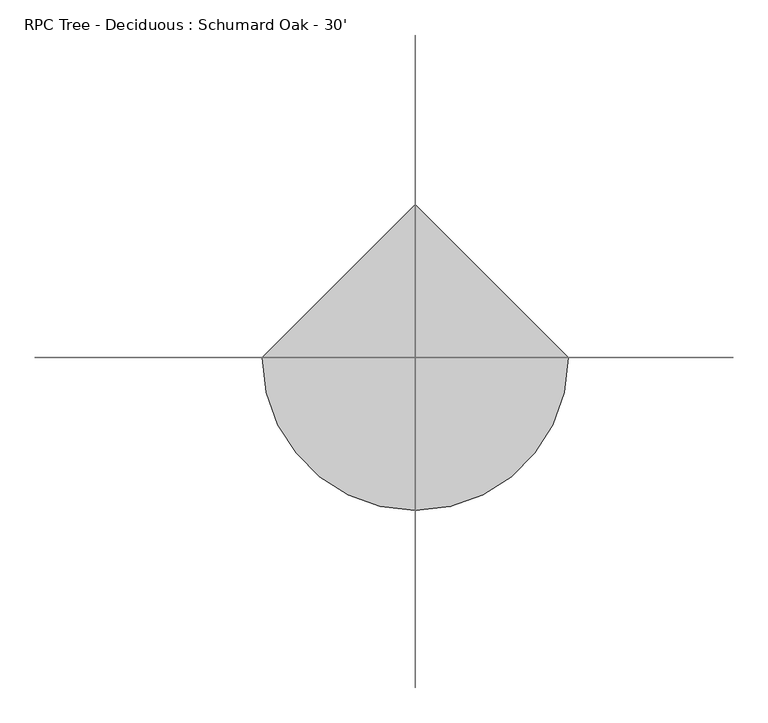
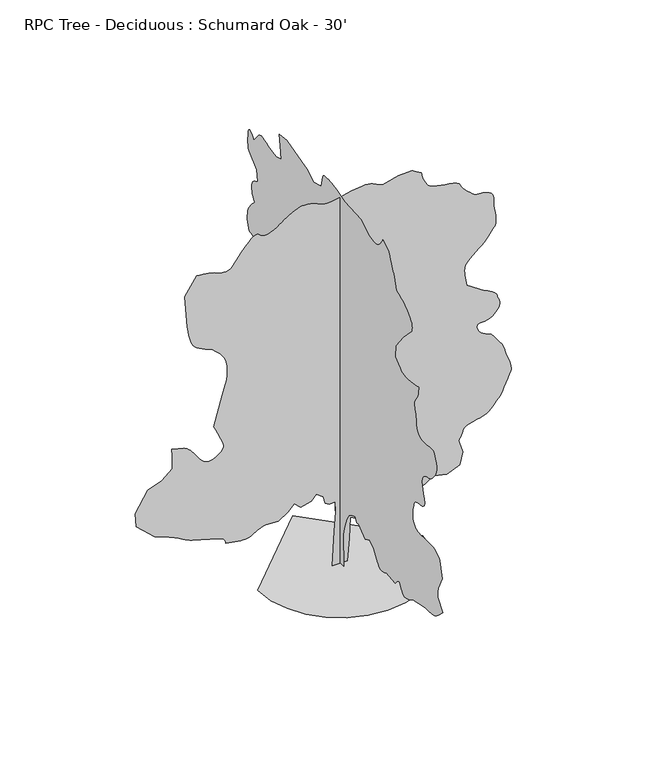
"""IFC4 building model written with IfcOpenShell, lengths in millimetres: geographic element geometry, RPC Tree - Deciduous : Schumard Oak - 30'."""

from ifc_helpers import new_model, si_unit, origin, place, context, project, spatial, triangles, source, transform, mapped, element, save


def rpc_tree_deciduous_schumard_oak_30_cf07c7db(model_context):
    return source(origin(), model_context, "Body", "Tessellation", [
        triangles([(-0.0016958, 164.6246354, 0.0086022), (-0.0016958, -151.6104316, 0.0086022), (-0.0016958, -124.1113561, 783.7227293), (-0.0016958, -179.1089983, 1017.4612965), (-0.0016958, -261.6049622, 1237.4509209), (-0.0016958, -357.8507226, 1388.6927067), (-0.0016958, -467.8454985, 1457.4403999), (-0.0016958, -605.3383779, 1512.436607), (-0.0016958, -660.3370193, 1388.6927067), (-0.0016958, -756.5828161, 1416.1908829), (-0.0016958, -866.5775557, 1306.195998), (-0.0016958, -1017.8194868, 1209.9502739), (-0.0016958, -1196.5619196, 1292.4469826), (-0.0016958, -1361.5527935, 1182.452243), (-0.0016958, -1471.5476784, 989.9607222), (-0.0016958, -1498.1643677, 951.9597713), (-0.0016958, -1525.3829098, 915.7621988), (-0.0016958, -1553.8031227, 883.1739264), (-0.0016958, -1584.0290394, 855.9959341), (-0.0016958, -1616.658007, 836.0340712), (-0.0016958, -1652.2942039, 825.0891724), (-0.0016958, -1691.5371574, 824.9697756), (-0.0016958, -1729.1774471, 831.662681), (-0.0016958, -1760.3255459, 839.8008471), (-0.0016958, -1786.0582775, 849.1404659), (-0.0016958, -1807.4654011, 859.4426714), (-0.0016958, -1825.6238857, 870.4663445), (-0.0016958, -1841.6182583, 881.9725462), (-0.0016958, -1856.5307201, 893.7149254), (-0.0016958, -2214.0131149, 852.4678791), (-0.0016958, -2249.2480282, 893.1561659), (-0.0016958, -2283.7616192, 930.4738735), (-0.0016958, -2316.8324203, 961.0605967), (-0.0016958, -2347.7391094, 981.54314), (-0.0016958, -2375.7578934, 988.5586275), (-0.0016958, -2400.1697754, 978.7389507), (-0.0016958, -2420.2535786, 948.7136032), (-0.0016958, -2440.416156, 905.5412384), (-0.0016958, -2465.389341, 860.9260838), (-0.0016958, -2494.9323051, 818.4750412), (-0.0016958, -2528.8058189, 781.7974108), (-0.0016958, -2566.7735596, 754.4999491), (-0.0016958, -2608.5820541, 740.1896307), (-0.0016958, -2653.9973053, 742.4730669), (-0.0016958, -2699.5395836, 755.8614212), (-0.0016958, -2742.1861084, 772.1352098), (-0.0016958, -2782.4196991, 790.8169184), (-0.0016958, -2820.7484642, 811.421402), (-0.0016958, -2857.6293526, 833.4686754), (-0.0016958, -2893.5448929, 856.475992), (-0.0016958, -2928.9779045, 879.96591), (-0.0016958, -3423.9482735, 976.2117067), (-0.0016958, -3485.6956673, 976.3335743), (-0.0016958, -3546.579451, 977.174366), (-0.0016958, -3605.7868835, 979.4603456), (-0.0016958, -3662.4543549, 983.9078939), (-0.0016958, -3715.7688332, 991.2459635), (-0.0016958, -3764.8925789, 1002.1882462), (-0.0016958, -3808.9361115, 1017.4612965), (-0.0016958, -3851.3797417, 1039.546649), (-0.0016958, -3896.0075409, 1069.5719965), (-0.0016958, -3942.4134293, 1106.2115479), (-0.0016958, -3990.2924835, 1148.1393665), (-0.0016958, -4039.2383331, 1194.0371464), (-0.0016958, -4088.8951859, 1242.5817123), (-0.0016958, -4138.9334106, 1292.4469826), (-0.0016958, -3946.4265564, 1512.436607), (-0.0016958, -3940.7114983, 1553.6455742), (-0.0016958, -3935.9362083, 1594.6132771), (-0.0016958, -3933.0916145, 1635.0983059), (-0.0016958, -3933.1169037, 1674.8646286), (-0.0016958, -3937.0032944, 1713.6657486), (-0.0016958, -3945.7152626, 1751.2679592), (-0.0016958, -3960.1934486, 1787.4247639), (-0.0016958, -4111.425206, 2103.6601124), (-0.0016958, -4015.1842781, 2488.640538), (-0.0016958, -4007.6405525, 2499.2628548), (-0.0016958, -3985.1869812, 2526.4815422), (-0.0016958, -3948.0776184, 2563.3191193), (-0.0016958, -3896.5156494, 2602.8164177), (-0.0016958, -3830.780127, 2637.9697952), (-0.0016958, -3751.1003975, 2661.820665), (-0.0016958, -3657.7046448, 2667.3831161), (-0.0016958, -3553.6406479, 2663.0650658), (-0.0016958, -3446.4524231, 2661.3634254), (-0.0016958, -3343.1000107, 2661.617189), (-0.0016958, -3250.5928665, 2663.0650658), (-0.0016958, -3175.8660324, 2664.970182), (-0.0016958, -3125.9298363, 2666.6718224), (-0.0016958, -3107.7178665, 2667.3831161), (-0.0016958, -3097.049913, 2674.6474983), (-0.0016958, -3069.5669975, 2695.1200859), (-0.0016958, -3031.9495262, 2726.9207611), (-0.0016958, -2990.9793526, 2768.0688309), (-0.0016958, -2953.3874611, 2816.7097572), (-0.0016958, -2925.9045456, 2870.8625565), (-0.0016958, -2915.2365921, 2928.622403), (-0.0016958, -2917.2431557, 2986.3310898), (-0.0016958, -2922.8564758, 3041.9064766), (-0.0016958, -2931.4672874, 3095.6529053), (-0.0016958, -2942.4907425, 3147.977037), (-0.0016958, -2955.3178665, 3199.2087936), (-0.0016958, -2969.3385223, 3249.7039673), (-0.0016958, -2983.9690247, 3299.8436394), (-0.0016958, -2996.0086967, 3314.52472), (-0.0016958, -3009.4706657, 3328.8250099), (-0.0016958, -3025.8280975, 3342.414006), (-0.0016958, -3046.5038704, 3354.9362068), (-0.0016958, -3072.9705688, 3365.9852417), (-0.0016958, -3106.6510712, 3375.2561874), (-0.0016958, -3148.9673836, 3382.3429642), (-0.0016958, -3200.1485619, 3386.6863037), (-0.0016958, -3255.4443146, 3391.740937), (-0.0016958, -3308.7843727, 3403.2725006), (-0.0016958, -3354.1996239, 3427.0722107), (-0.0016958, -3385.6703773, 3468.9315742), (-0.0016958, -3397.1766518, 3534.5906479), (-0.0016958, -3382.6984657, 3629.8406479), (-0.0016958, -3353.0819595, 3737.5114014), (-0.0016958, -3325.8786781, 3836.2667107), (-0.0016958, -3305.152327, 3925.6746254), (-0.0016958, -3294.9921913, 4005.2023293), (-0.0016958, -3299.5387161, 4074.3920013), (-0.0016958, -3322.8306084, 4132.761113), (-0.0016958, -3368.9571533, 4179.8018463), (-0.0016958, -3425.5228867, 4212.7710548), (-0.0016958, -3477.9993347, 4232.964299), (-0.0016958, -3527.3262657, 4246.1975029), (-0.0016958, -3574.5193153, 4258.2118858), (-0.0016958, -3620.493544, 4274.8233719), (-0.0016958, -3666.2390076, 4301.7473099), (-0.0016958, -3712.6954742, 4344.8004959), (-0.0016958, -3760.0411308, 4399.562851), (-0.0016958, -3805.2023277, 4457.9322533), (-0.0016958, -3844.3694138, 4520.1368866), (-0.0016958, -3873.6809967, 4586.4308052), (-0.0016958, -3889.2765564, 4657.068354), (-0.0016958, -3887.295282, 4732.2777168), (-0.0016958, -3863.9272316, 4812.2879494), (-0.0016958, -3835.7077332, 4887.9545517), (-0.0016958, -3816.632444, 4949.7019455), (-0.0016958, -3799.0047409, 4996.9967331), (-0.0016958, -3775.1032928, 5029.3819656), (-0.0016958, -3737.2573471, 5046.3745331), (-0.0016958, -3677.7705711, 5047.4919067), (-0.0016958, -3588.9466324, 5032.2771378), (-0.0016958, -3483.5620766, 5015.437468), (-0.0016958, -3382.266806, 5012.0591858), (-0.0016958, -3289.150106, 5022.1684525), (-0.0016958, -3208.3018433, 5045.7396881), (-0.0016958, -3143.7860138, 5082.7728928), (-0.0016958, -3099.7421906, 5133.2930649), (-0.0016958, -3080.2096619, 5197.2507889), (-0.0016958, -3073.5295464, 5265.5768509), (-0.0016958, -3065.4015541, 5329.5339935), (-0.0016958, -3056.0541595, 5389.9099594), (-0.0016958, -3045.7417076, 5447.3901718), (-0.0016958, -3034.7182526, 5502.7112137), (-0.0016958, -3023.2119781, 5556.5846695), (-0.0016958, -3011.4772293, 5609.7471222), (-0.0016958, -3000.047113, 5648.0755966), (-0.0016958, -2990.8014565, 5686.505809), (-0.0016958, -2985.8485611, 5725.1900757), (-0.0016958, -2987.423465, 5764.2295532), (-0.0016958, -2997.6341789, 5803.7521408), (-0.0016958, -3018.6907425, 5843.8839935), (-0.0016958, -3052.7267464, 5884.7274307), (-0.0016958, -3089.125106, 5934.8418137), (-0.0016958, -3116.6080215, 5997.6815826), (-0.0016958, -3136.4198936, 6065.8297485), (-0.0016958, -3149.7295464, 6131.8187439), (-0.0016958, -3157.7558006, 6188.1815826), (-0.0016958, -3161.6674805, 6227.450116), (-0.0016958, -3162.7089867, 6242.2073547), (-0.0016958, -3142.4395844, 6237.6861191), (-0.0016958, -3088.0074417, 6226.1798447), (-0.0016958, -3009.0387154, 6210.8383392), (-0.0016958, -2915.160434, 6194.7602509), (-0.0016958, -2815.9731743, 6181.0948059), (-0.0016958, -2721.1295448, 6172.9418152), (-0.0016958, -2640.2304131, 6173.4749222), (-0.0016958, -2571.9299309, 6185.3619873), (-0.0016958, -2507.9599983, 6208.094902), (-0.0016958, -2447.5915901, 6239.8452896), (-0.0016958, -2390.1089069, 6278.808609), (-0.0016958, -2334.7901905, 6323.1826447), (-0.0016958, -2280.9167347, 6371.1634369), (-0.0016958, -2227.7621304, 6420.9476074), (-0.0016958, -2241.5111458, 6709.6945175), (-0.0016958, -2543.9897758, 7094.6826462), (-0.0016958, -2887.7283875, 7452.1625702), (-0.0016958, -2893.1132332, 7496.4860275), (-0.0016958, -2895.3482712, 7541.6722229), (-0.0016958, -2891.335144, 7588.5356415), (-0.0016958, -2877.9493332, 7637.9128601), (-0.0016958, -2852.0666107, 7690.6689423), (-0.0016958, -2810.5377502, 7747.6160477), (-0.0016958, -2750.2379425, 7809.6424942), (-0.0016958, -2679.5242355, 7869.2562973), (-0.0016958, -2608.8108192, 7919.4724182), (-0.0016958, -2538.10467, 7961.8901779), (-0.0016958, -2467.3935791, 7998.0344833), (-0.0016958, -2396.6824883, 8029.5052368), (-0.0016958, -2325.9712521, 8057.8517624), (-0.0016958, -2255.2601612, 8084.6233841), (-0.0016958, -2234.6175259, 8155.1336151), (-0.0016958, -2213.8530956, 8224.4503143), (-0.0016958, -2192.8472557, 8291.3537888), (-0.0016958, -2171.4808273, 8354.651088), (-0.0016958, -2149.6341957, 8413.1219376), (-0.0016958, -2127.1881821, 8465.5983856), (-0.0016958, -2104.0183754, 8510.8607391), (-0.0016958, -2078.3235775, 8560.2129593), (-0.0016958, -2049.9822842, 8621.0970337), (-0.0016958, -2021.4021973, 8686.5529221), (-0.0016958, -1994.9862225, 8749.5955856), (-0.0016958, -1973.1395908, 8803.2917267), (-0.0016958, -1958.2679695, 8840.6039841), (-0.0016958, -1952.7738281, 8854.5996414), (-0.0016958, -1719.0353336, 8992.089505), (-0.0016958, -1707.0516174, 8968.3915329), (-0.0016958, -1693.863905, 8943.9819763), (-0.0016958, -1678.2681999, 8918.1248337), (-0.0016958, -1659.0683544, 8890.1085205), (-0.0016958, -1635.057756, 8859.1970352), (-0.0016958, -1605.0324085, 8824.678212), (-0.0016958, -1567.7934025, 8785.841629), (-0.0016958, -1522.9369835, 8752.2122864), (-0.0016958, -1471.5882282, 8732.2983856), (-0.0016958, -1414.8268673, 8723.7896027), (-0.0016958, -1353.7372822, 8724.4244476), (-0.0016958, -1289.3990582, 8731.9175949), (-0.0016958, -1222.896722, 8743.9825562), (-0.0016958, -1155.3123299, 8758.3334244), (-0.0016958, -852.8259968, 8964.5813004), (-0.0016958, -192.8582863, 9005.8311081), (-0.0016958, -107.5965211, 9029.2756073), (-0.0016958, -23.416737, 9052.008522), (-0.0016958, 58.5983536, 9073.2938507), (-0.0016958, 137.366361, 9092.4200089), (-0.0016958, 211.8051857, 9108.6504135), (-0.0016958, 280.8327856, 9121.2740616), (-0.0016958, 343.3650879, 9129.57995), (-0.0016958, 405.0185557, 9135.9045639), (-0.0016958, 469.5549508, 9141.5181747), (-0.0016958, 533.1311937, 9144.0075577), (-0.0016958, 591.8966838, 9140.9594879), (-0.0016958, 642.0033274, 9129.9863205), (-0.0016958, 679.6029219, 9108.6504135), (-0.0016958, 700.8500261, 9074.5891205), (-0.0016958, 769.5952486, 8799.5832321), (-0.0016958, 1072.081509, 8717.1091965), (-0.0016958, 1347.0698112, 8882.0822662), (-0.0016958, 1690.8031906, 8964.5813004), (-0.0016958, 2144.5313095, 9102.0717453), (-0.0016958, 2447.0174973, 9060.8225189), (-0.0016958, 2419.5169956, 8799.5832321), (-0.0016958, 2364.5209339, 8497.1197174), (-0.0016958, 2584.5030006, 8428.361705), (-0.0016958, 2804.4924797, 8469.6115128), (-0.0016958, 2889.5570549, 8501.5647949), (-0.0016958, 2972.3357231, 8530.7490601), (-0.0016958, 3050.5425774, 8554.3964539), (-0.0016958, 3121.8911293, 8569.7385406), (-0.0016958, 3184.1210518, 8574.0307205), (-0.0016958, 3234.8958595, 8564.480722), (-0.0016958, 3271.9799332, 8538.3439453), (-0.0016958, 3478.2280998, 8290.8712601), (-0.0016958, 3525.090937, 8345.6591949), (-0.0016958, 3570.2521339, 8393.3603531), (-0.0016958, 3612.0606285, 8426.8885391), (-0.0016958, 3648.8144897, 8439.1058167), (-0.0016958, 3678.8373665, 8422.9515701), (-0.0016958, 3700.4526169, 8371.313443), (-0.0016958, 3711.9588913, 8277.1046585), (-0.0016958, 3715.4389114, 8172.4819748), (-0.0016958, 3714.6005905, 8091.684581), (-0.0016958, 3710.155513, 8030.6987686), (-0.0016958, 3702.8149727, 7985.6137299), (-0.0016958, 3693.3152618, 7952.4163376), (-0.0016958, 3682.3679649, 7927.1684601), (-0.0016958, 3670.7093742, 7905.8831314), (-0.0016958, 3354.4789673, 7644.6438446), (-0.0016958, 3326.9707626, 7355.921933), (-0.0016958, 3370.9384277, 7337.989888), (-0.0016958, 3413.6102417, 7318.6346741), (-0.0016958, 3453.615358, 7296.384288), (-0.0016958, 3489.6326363, 7269.8161423), (-0.0016958, 3520.3920959, 7237.4564896), (-0.0016958, 3544.5220184, 7197.8833237), (-0.0016958, 3560.7018448, 7149.674057), (-0.0016958, 3566.8994316, 7096.6389221), (-0.0016958, 3562.9624626, 7043.6032059), (-0.0016958, 3550.618158, 6990.568071), (-0.0016958, 3531.5425781, 6937.5329361), (-0.0016958, 3507.4126556, 6884.4978012), (-0.0016958, 3479.904451, 6831.4626663), (-0.0016958, 3450.7198952, 6778.4269501), (-0.0016958, 3494.7381386, 6734.2313919), (-0.0016958, 3537.6640068, 6689.8829361), (-0.0016958, 3578.4309952, 6645.3060059), (-0.0016958, 3615.9470192, 6600.3732834), (-0.0016958, 3649.1447021, 6554.9580322), (-0.0016958, 3676.9322502, 6508.9329346), (-0.0016958, 3698.2175789, 6462.1968338), (-0.0016958, 3713.4829262, 6416.6548462), (-0.0016958, 3724.4305138, 6374.0080307), (-0.0016958, 3731.7710541, 6333.77444), (-0.0016958, 3736.2161316, 6295.4459656), (-0.0016958, 3738.5020386, 6258.5650772), (-0.0016958, 3739.3400688, 6222.6492462), (-0.0016958, 3739.4670959, 6187.2165253), (-0.0016958, 3656.9680618, 5953.4854431), (-0.0016958, 3618.6901657, 5947.3387253), (-0.0016958, 3580.5140076, 5939.7694199), (-0.0016958, 3542.591613, 5929.304361), (-0.0016958, 3505.0250107, 5914.5215424), (-0.0016958, 3467.9665169, 5893.9477982), (-0.0016958, 3431.4664192, 5866.1599594), (-0.0016958, 3395.728775, 5829.7366013), (-0.0016958, 3363.165937, 5786.4799393), (-0.0016958, 3335.6830215, 5739.6171021), (-0.0016958, 3312.3911293, 5689.7567734), (-0.0016958, 3292.4522301, 5637.4838013), (-0.0016958, 3275.0532921, 5583.4068695), (-0.0016958, 3259.3559944, 5528.1364059), (-0.0016958, 3244.4717285, 5472.2566772), (-0.0016958, 3212.2896812, 5428.0349579), (-0.0016958, 3181.4287743, 5383.7120819), (-0.0016958, 3153.2092758, 5339.1351517), (-0.0016958, 3128.9523262, 5294.1768494), (-0.0016958, 3110.0037735, 5248.7615982), (-0.0016958, 3097.6341797, 5202.7620804), (-0.0016958, 3093.2399712, 5156.026561), (-0.0016958, 3106.9812836, 4784.7797447), (-0.0016958, 3139.1630402, 4781.5284897), (-0.0016958, 3170.049527, 4776.4738564), (-0.0016958, 3198.2690254, 4767.8377556), (-0.0016958, 3222.5006859, 4753.7662308), (-0.0016958, 3241.4745277, 4732.4809021), (-0.0016958, 3253.8188324, 4702.1533928), (-0.0016958, 3258.2383301, 4661.0306122), (-0.0016958, 3257.0192184, 4613.5073502), (-0.0016958, 3253.6665161, 4565.2219254), (-0.0016958, 3248.4848557, 4516.377523), (-0.0016958, 3241.8808983, 4467.0253029), (-0.0016958, 3234.1845657, 4417.3175812), (-0.0016958, 3225.7516502, 4367.3810944), (-0.0016958, 3216.988813, 4317.2922913), (-0.0016958, 3203.2219208, 4042.311692), (-0.0016958, 3464.4612076, 4056.0785843), (-0.0016958, 3753.208699, 4111.0694138), (-0.0016958, 3814.6511696, 4090.2669044), (-0.0016958, 3873.5792587, 4068.37202), (-0.0016958, 3927.4527145, 4044.3182556), (-0.0016958, 3973.7568649, 4017.0132362), (-0.0016958, 4009.9520393, 3985.3901665), (-0.0016958, 4033.523275, 3948.3569618), (-0.0016958, 4041.9306107, 3904.8212471), (-0.0016958, 4039.5429657, 3849.6778107), (-0.0016958, 4032.8119812, 3780.081768), (-0.0016958, 4022.448951, 3698.4716331), (-0.0016958, 4009.2407455, 3607.2347603), (-0.0016958, 3993.8483711, 3508.7840836), (-0.0016958, 3977.00812, 3405.5078293), (-0.0016958, 3959.4568657, 3299.8436394), (-0.0016958, 3835.7077332, 2969.87192), (-0.0016958, 3768.1185448, 2931.9498161), (-0.0016958, 3701.6211502, 2896.3136192), (-0.0016958, 3637.2829262, 2865.2492363), (-0.0016958, 3576.1959572, 2841.0431557), (-0.0016958, 3519.4267479, 2825.9554138), (-0.0016958, 3468.0679642, 2822.3233681), (-0.0016958, 3423.2113998, 2832.3817657), (-0.0016958, 3038.248851, 2997.3548355), (-0.0016958, 2653.2607224, 2873.6312828), (-0.0016958, 2378.2699493, 2681.1244286), (-0.0016958, 2103.2842632, 2268.651059), (-0.0016958, 2076.6675739, 2227.6428062), (-0.0016958, 2049.4488865, 2188.0796688), (-0.0016958, 2021.0263481, 2151.4021111), (-0.0016958, 1990.8027569, 2119.0526321), (-0.0016958, 1958.1739346, 2092.4764927), (-0.0016958, 1922.5377377, 2073.1141571), (-0.0016958, 1883.2946388, 2062.4105953), (-0.0016958, 1844.1303143, 2058.8443886), (-0.0016958, 1807.3715115, 2059.123732), (-0.0016958, 1770.371299, 2062.0498615), (-0.0016958, 1730.4881229, 2066.4186356), (-0.0016958, 1685.070401, 2071.0288193), (-0.0016958, 1631.4762886, 2074.6762711), (-0.0016958, 1567.0592903, 2076.1596107), (-0.0016958, 1497.9510086, 2070.950045), (-0.0016958, 1431.730632, 2056.3577671), (-0.0016958, 1367.9130157, 2033.9498325), (-0.0016958, 1306.020718, 2005.2883553), (-0.0016958, 1245.5712101, 1971.9382107), (-0.0016958, 1186.0844341, 1935.4612221), (-0.0016958, 1127.0801868, 1897.4196487), (-0.0016958, 1044.5834782, 1663.6810089), (-0.0016958, 810.8448383, 1402.4418674), (-0.0016958, 778.5741337, 1367.4862976), (-0.0016958, 741.256426, 1333.2546661), (-0.0016958, 699.7273476, 1299.622562), (-0.0016958, 654.8303061, 1266.4729866), (-0.0016958, 607.408455, 1233.6815289), (-0.0016958, 558.3051295, 1201.1339516), (-0.0016958, 508.3585416, 1168.7032276), (-0.0016958, 425.8618329, 1457.4403999), (-0.0016958, 288.3689717, 1649.9293774), (-0.0016958, 233.3715837, 1526.1856224), (-0.0016958, 192.1232112, 1333.696645), (-0.0016958, 178.3741776, 989.9607222), (-0.0016958, 150.8753565, 508.7344634), (170.3625119, 0.000436, 0.0217742), (-187.1199193, 0.000436, 0.0217742), (-132.1230309, 0.000387, 824.9824928), (-104.6242098, 0.0003581, 1306.2087879), (-118.3734886, 0.0003434, 1553.698914), (-255.8671038, 0.0003442, 1539.9498985), (-352.1128461, 0.000341, 1594.9459602), (-393.359965, 0.0003302, 1773.6885384), (-558.3534187, 0.0003237, 1883.6832779), (-668.3482309, 0.000331, 1759.9395229), (-915.8358135, 0.0003352, 1691.1918297), (-1067.0802881, 0.0003271, 1828.6846001), (-1218.3221466, 0.000336, 1677.4428143), (-1438.311771, 0.0003442, 1539.9498985), (-1768.2961349, 0.0003434, 1553.698914), (-1933.2869362, 0.0003476, 1484.9512207), (-1968.7250347, 0.0003491, 1458.6138748), (-2004.6407204, 0.0003507, 1433.3612011), (-2041.5189926, 0.000352, 1410.2726395), (-2079.8425255, 0.0003531, 1390.4301006), (-2120.0889061, 0.0003541, 1374.915786), (-2162.738047, 0.0003547, 1364.8142223), (-2208.2752384, 0.0003549, 1361.2074657), (-2259.0244663, 0.0003549, 1362.8101295), (-2316.2658852, 0.0003547, 1367.3008438), (-2378.9175842, 0.0003541, 1374.1944637), (-2445.902449, 0.0003536, 1383.0132568), (-2516.1310112, 0.0003531, 1393.2749851), (-2588.5161278, 0.0003523, 1404.4991547), (-2661.9982704, 0.0003518, 1416.2061436), (-2665.4018417, 0.0003499, 1445.5887978), (-2671.5741394, 0.0003481, 1474.4889233), (-2683.2835991, 0.0003465, 1502.428933), (-2703.2986565, 0.0003449, 1528.9262981), (-2734.3630394, 0.0003434, 1553.4981995), (-2779.2448929, 0.0003421, 1575.6648697), (-2840.7382324, 0.000341, 1594.9459602), (-3445.7158401, 0.0003302, 1773.6885384), (-3495.0936401, 0.0003295, 1789.3602562), (-3547.8494316, 0.0003281, 1811.5293972), (-3602.2815742, 0.0003266, 1838.265556), (-3656.7140076, 0.0003247, 1867.6482101), (-3709.469799, 0.0003229, 1897.7523319), (-3758.8728882, 0.0003213, 1926.6550735), (-3803.1957642, 0.0003197, 1952.4285004), (-3850.8716331, 0.0003182, 1977.2011162), (-3910.0790657, 0.0003166, 2004.1403149), (-3978.8876564, 0.0003148, 2032.8804211), (-4055.4181595, 0.0003132, 2063.0657879), (-4137.7140083, 0.0003113, 2094.3332108), (-4223.8456696, 0.0003092, 2126.3194851), (-4311.9327347, 0.0003074, 2158.668964), (-4738.1450912, 0.0002835, 2557.4011665), (-4765.6532959, 0.0002638, 2887.3725952), (-4476.9060951, 0.000236, 3354.8600487), (-4146.9343758, 0.0002287, 3478.6088905), (-3899.4364014, 0.0002163, 3684.8570572), (-3899.4364014, 0.0001977, 4001.0874641), (-3913.2032936, 0.0001877, 4166.0858231), (-3624.4558022, 0.0001919, 4097.3281013), (-3591.9438332, 0.0001932, 4076.3729851), (-3558.8475975, 0.0001945, 4053.3607269), (-3524.5322502, 0.0001961, 4026.2588928), (-3488.4135246, 0.0001979, 3993.03563), (-3449.8815742, 0.0002006, 3951.6082169), (-3408.3524231, 0.0002037, 3899.9953789), (-3363.216806, 0.0002074, 3836.0888145), (-3317.4713425, 0.0002113, 3768.956575), (-3273.4275192, 0.000215, 3709.7491425), (-3229.3839867, 0.0002179, 3659.6856285), (-3183.6385231, 0.0002203, 3619.9601463), (-3134.5403572, 0.0002221, 3591.765937), (-3080.387558, 0.0002229, 3576.3482735), (-3019.4781944, 0.0002229, 3574.8495277), (-2952.9046417, 0.0002221, 3590.0895859), (-2885.848851, 0.0002203, 3620.9507835), (-2822.8567657, 0.0002176, 3662.8860146), (-2768.5513596, 0.0002147, 3711.2984665), (-2727.4541588, 0.0002119, 3761.6413239), (-2704.1622665, 0.000209, 3809.3427727), (-2703.2480782, 0.0002066, 3849.8304176), (-2719.4531937, 0.000204, 3893.6198959), (-2743.5831161, 0.0002006, 3952.5479851), (-2774.3172867, 0.0001961, 4024.0997223), (-2810.3598541, 0.0001914, 4105.735437), (-2850.3649704, 0.0001861, 4194.9657463), (-2893.0114952, 0.0001803, 4289.2506889), (-2936.9788696, 0.0001746, 4386.0755928), (-2744.4975952, 0.0001328, 5087.2685486), (-2718.1576332, 0.0001281, 5166.6433548), (-2692.9100464, 0.0001234, 5244.9263672), (-2669.8216301, 0.0001189, 5321.050209), (-2649.9841782, 0.0001145, 5393.948085), (-2634.4647766, 0.0001105, 5462.477623), (-2624.3555099, 0.0001066, 5525.6220245), (-2620.7487534, 0.0001034, 5582.263916), (-2621.6885216, 0.0001, 5637.5343796), (-2624.7618805, 9.66e-05, 5696.1831253), (-2630.5022278, 9.29e-05, 5756.5079315), (-2639.366803, 8.93e-05, 5816.8333191), (-2651.8128456, 8.58e-05, 5875.4820648), (-2668.3737534, 8.24e-05, 5930.7525284), (-2689.5064751, 7.95e-05, 5980.9936478), (-2716.6844673, 7.67e-05, 6027.7297485), (-2750.3649696, 7.4e-05, 6073.7542648), (-2789.4303177, 7.14e-05, 6119.169516), (-2832.8390053, 6.85e-05, 6164.1022385), (-2879.4986572, 6.59e-05, 6208.6791687), (-2928.3430595, 6.33e-05, 6253.002626), (-2978.2286774, 6.06e-05, 6297.223764), (-3057.4511673, 5.88e-05, 6329.6851547), (-3134.6165154, 5.67e-05, 6362.5273361), (-3207.6922874, 5.49e-05, 6396.0805206), (-3274.6213417, 5.28e-05, 6430.7010818), (-3333.3971146, 5.07e-05, 6466.7942276), (-3381.9365936, 4.83e-05, 6504.6657532), (-3418.2076355, 4.59e-05, 6544.7214478), (-3446.7573463, 4.28e-05, 6598.1123749), (-3473.1478867, 3.86e-05, 6670.5027237), (-3496.8717293, 3.36e-05, 6753.9668152), (-3517.4710533, 2.84e-05, 6840.5557159), (-3534.4636208, 2.34e-05, 6922.3181671), (-3547.3669029, 1.94e-05, 6991.3558136), (-3555.7233696, 1.65e-05, 7039.6918167), (-3610.7144897, -2.94e-05, 7809.6424942), (-3335.7086014, -5.49e-05, 8235.8804306), (-3262.2517479, -5.43e-05, 8226.9396973), (-3189.8616898, -5.38e-05, 8217.4146973), (-3119.6305115, -5.3e-05, 8206.6705856), (-3052.6252991, -5.22e-05, 8194.1225143), (-2989.9887154, -5.15e-05, 8179.162381), (-2932.7372681, -5.04e-05, 8161.2041748), (-2881.9880402, -4.91e-05, 8139.6397934), (-2830.4004913, -4.78e-05, 8118.7864151), (-2772.3107231, -4.7e-05, 8104.2064911), (-2711.3504906, -4.65e-05, 8097.069136), (-2651.1018425, -4.67e-05, 8098.5934616), (-2595.1709541, -4.73e-05, 8109.9724182), (-2547.1901619, -4.86e-05, 8132.4262802), (-2510.7589554, -5.07e-05, 8167.1224182), (-2290.7694763, -6.8e-05, 8455.8699097), (-2232.0038773, -7.19e-05, 8523.1291763), (-2174.2011555, -7.59e-05, 8587.3915329), (-2118.3236069, -7.93e-05, 8645.6333267), (-2065.3290218, -8.22e-05, 8694.8588104), (-2016.1850739, -8.45e-05, 8732.0699112), (-1971.8492626, -8.58e-05, 8754.2185593), (-1933.2869362, -8.61e-05, 8758.3590042), (-1902.260923, -8.53e-05, 8748.0212631), (-1877.0081039, -8.43e-05, 8731.181012), (-1853.1982201, -8.32e-05, 8711.4450073), (-1826.5002857, -8.22e-05, 8692.4455856), (-1792.5886929, -8.11e-05, 8677.7900848), (-1747.1302757, -8.09e-05, 8671.0591003), (-1685.7992809, -8.11e-05, 8675.8593887), (-1612.5227943, -8.24e-05, 8696.712767), (-1537.32346, -8.43e-05, 8731.5112244), (-1465.0070892, -8.69e-05, 8773.9795624), (-1400.3895218, -8.95e-05, 8817.9216476), (-1348.2787491, -9.19e-05, 8857.0378647), (-1313.4833439, -9.35e-05, 8885.1047562), (-1300.8163845, -9.42e-05, 8895.8488678), (-1285.3045406, -9.48e-05, 8905.7802383), (-1244.0574944, -9.63e-05, 8931.6123825), (-1185.0100084, -9.84e-05, 8967.2741592), (-1116.1022959, -0.0001008, 9006.7961655), (-1045.2718082, -0.0001029, 9044.1595825), (-980.4534536, -0.0001047, 9073.344429), (-929.5848289, -0.0001055, 9088.3307236), (-881.3222952, -0.0001058, 9091.6578461), (-821.2740709, -0.0001058, 9089.7021515), (-752.8083372, -0.0001053, 9082.2090042), (-679.2905136, -0.0001045, 9068.9505112), (-604.0912156, -0.0001034, 9049.6714554), (-530.573392, -0.0001019, 9024.1189453), (-462.1076583, -0.0001, 8992.089505), (-389.2730779, -9.84e-05, 8965.9533096), (-302.0062388, -9.79e-05, 8956.4283096), (-202.713753, -9.79e-05, 8960.7204895), (-93.8012603, -9.9e-05, 8976.0625763), (22.3266441, -0.0001003, 8999.7099701), (143.2647473, -0.0001021, 9028.8942352), (266.608781, -0.000104, 9060.8475174), (351.7496415, -0.0001047, 9072.3793716), (435.0871056, -0.0001053, 9082.4886383), (514.8177767, -0.0001058, 9089.7021515), (589.1356968, -0.0001058, 9092.597905), (656.2400311, -0.0001058, 9089.7021515), (714.324785, -0.000105, 9079.5928848), (761.584037, -0.000104, 9060.8475174), (801.2284195, -0.0001026, 9038.8767654), (837.987295, -0.0001016, 9019.8011856), (872.3408667, -0.0001005, 9003.1132507), (904.7690472, -9.98e-05, 8988.356012), (935.7570539, -9.9e-05, 8975.0719391), (965.779858, -9.82e-05, 8962.7017639), (995.3226768, -9.74e-05, 8950.8402786), (1352.8050716, -0.0001032, 9047.0809158), (1669.0404202, -0.000104, 9060.8475174), (1889.0325153, -9.66e-05, 8937.0986755), (1892.1974384, -9.48e-05, 8904.5611267), (1896.6881527, -9.27e-05, 8871.1602585), (1903.8228916, -9.06e-05, 8836.0827484), (1914.9278824, -8.85e-05, 8798.4908569), (1931.3210678, -8.58e-05, 8757.5206833), (1954.3308552, -8.32e-05, 8712.3339066), (1985.2757687, -8.03e-05, 8662.118367), (2016.3831722, -7.74e-05, 8616.1438477), (2042.1971489, -7.56e-05, 8582.1842926), (2067.531213, -7.4e-05, 8557.1398911), (2097.1958267, -7.27e-05, 8537.8358368), (2135.9969467, -7.19e-05, 8521.1990616), (2188.7502674, -7.09e-05, 8504.1047562), (2260.2639256, -6.96e-05, 8483.3781143), (2348.4121788, -6.85e-05, 8463.4136353), (2443.5351517, -6.75e-05, 8448.2500259), (2539.1383278, -6.67e-05, 8434.3055283), (2628.7244293, -6.56e-05, 8417.9478058), (2705.8133286, -6.43e-05, 8395.5701019), (2763.9030968, -6.25e-05, 8363.5918213), (2796.4915146, -5.99e-05, 8318.3794647), (2820.5705681, -5.67e-05, 8265.7507004), (2856.206765, -5.36e-05, 8213.8329391), (2901.4696999, -5.04e-05, 8162.5250244), (2954.4286766, -4.75e-05, 8111.6996384), (3013.1535805, -4.44e-05, 8061.2300446), (3075.7137154, -4.15e-05, 8011.0139236), (3140.2298355, -3.83e-05, 7960.8995407), (3230.9333107, -3.78e-05, 7951.6035965), (3317.928582, -3.73e-05, 7939.5386353), (3397.4559952, -3.62e-05, 7921.9362213), (3465.8073463, -3.47e-05, 7896.027919), (3519.2235626, -3.23e-05, 7859.0708725), (3554.0217293, -2.94e-05, 7808.2966461), (3566.4421921, -2.55e-05, 7740.9100616), (3567.2549332, -2.13e-05, 7670.7044632), (3569.4902618, -1.76e-05, 7612.0812973), (3572.9447021, -1.47e-05, 7563.0337097), (3577.3641998, -1.23e-05, 7521.7077438), (3582.4949913, -1.02e-05, 7486.1732849), (3588.1086021, -8.1e-06, 7454.4484772), (3593.9503967, -6.6e-06, 7424.6799454), (3605.4566711, -2.4e-06, 7354.1947128), (3615.2865944, 1.8e-06, 7285.1832275), (3621.7382355, 5.8e-06, 7219.0413345), (3623.1352432, 9.5e-06, 7157.2177826), (3617.8009758, 1.29e-05, 7101.1851563), (3604.0596634, 1.58e-05, 7052.3666245), (3580.2090843, 1.81e-05, 7012.1836121), (3549.779837, 2.05e-05, 6973.6772415), (3516.9376556, 2.31e-05, 6929.6084198), (3480.9965355, 2.6e-05, 6881.221257), (3441.1948952, 2.89e-05, 6829.7098663), (3396.8208595, 3.2e-05, 6776.2933594), (3347.138427, 3.54e-05, 6722.1408508), (3291.4615929, 3.86e-05, 6668.4452911), (3226.8184456, 4.2e-05, 6613.0986694), (3154.6824417, 4.54e-05, 6553.8912369), (3081.1241409, 4.91e-05, 6492.0421051), (3012.1376541, 5.28e-05, 6428.7453873), (2953.7429626, 5.67e-05, 6365.2196136), (2911.9344681, 6.04e-05, 6302.6338989), (2892.7321518, 6.41e-05, 6242.2329346), (2889.6587929, 6.75e-05, 6182.4918137), (2891.6144875, 7.11e-05, 6121.3286865), (2897.7867851, 7.48e-05, 6058.9464478), (2907.3370743, 7.88e-05, 5995.6241501), (2919.4020355, 8.24e-05, 5931.5652695), (2933.1436386, 8.64e-05, 5867.0238602), (2947.7232719, 9.03e-05, 5802.2533951), (3360.2196053, 0.0001066, 5527.2475067), (3376.1959557, 0.0001071, 5520.1357315), (3417.4457634, 0.0001082, 5500.475885), (3473.8591805, 0.00011, 5470.9864059), (3535.3019417, 0.0001121, 5434.2584152), (3591.7153587, 0.0001147, 5392.9830276), (3632.9648758, 0.0001171, 5349.7525269), (3648.9415169, 0.0001197, 5307.2580276), (3657.5267487, 0.0001221, 5267.1511734), (3677.1610153, 0.0001244, 5227.0193207), (3698.7256874, 0.0001271, 5183.5347656), (3713.0765556, 0.0001302, 5133.2930649), (3711.0699921, 0.0001336, 5072.9682587), (3683.5870766, 0.0001381, 4999.1814835), (3621.4586014, 0.0001436, 4908.5282959), (3535.7588905, 0.0001481, 4831.4141075), (3447.6462456, 0.0001504, 4791.5613075), (3363.1403572, 0.0001515, 4775.7881424), (3288.2612068, 0.0001517, 4770.8096672), (3229.0029053, 0.0001523, 4763.4182579), (3191.4110138, 0.0001536, 4740.4312889), (3181.4796432, 0.0001567, 4688.5388168), (3195.7796425, 0.0001604, 4623.8450912), (3225.2438324, 0.0001635, 4569.9716354), (3267.3316704, 0.0001664, 4525.1153618), (3319.528775, 0.0001685, 4487.4723106), (3379.2948944, 0.0001704, 4455.2396851), (3444.1156471, 0.0001722, 4426.6393959), (3511.4510719, 0.0001738, 4399.8169052), (3578.7612076, 0.0001788, 4314.6761719), (3643.3026169, 0.0001838, 4231.3385262), (3702.3068642, 0.0001885, 4151.6079277), (3753.0055138, 0.000193, 4077.2874641), (3792.6548378, 0.0001972, 4010.1805138), (3818.4611115, 0.0002006, 3952.0907455), (3827.6814789, 0.0002032, 3904.8468269), (3838.9084099, 0.0002066, 3848.3063828), (3866.9753014, 0.0002116, 3767.5086983), (3903.4498192, 0.0002171, 3671.7761696), (3939.9240463, 0.0002231, 3570.531768), (3967.9912285, 0.0002289, 3473.1225975), (3979.2178688, 0.0002342, 3388.9469215), (3965.1716331, 0.0002378, 3327.351844), (3932.583506, 0.0002413, 3266.5442184), (3894.7119804, 0.0002462, 3184.3498169), (3852.9799347, 0.000252, 3089.6076347), (3808.8599533, 0.0002578, 2991.2842758), (3763.7496254, 0.0002633, 2898.2440247), (3719.1471153, 0.000268, 2819.4023254), (3676.4497215, 0.0002714, 2763.6493332), (3635.0475975, 0.0002741, 2719.4784828), (3592.6804161, 0.000277, 2671.193058), (3548.3828293, 0.0002798, 2621.4853363), (3501.189489, 0.0002827, 2572.9967262), (3450.1609177, 0.0002854, 2528.3384056), (3394.3317673, 0.0002877, 2490.1773628), (3332.7114006, 0.0002893, 2461.1552971), (3259.8893921, 0.0002906, 2439.6287041), (3175.9677704, 0.0002919, 2420.2688393), (3088.4646812, 0.000293, 2400.1850361), (3004.822403, 0.0002943, 2376.4944763), (2932.457634, 0.0002961, 2346.3115803), (2878.8638123, 0.0002985, 2306.7459721), (2851.4823441, 0.0003016, 2254.9146881), (2836.8265526, 0.0003048, 2202.96408), (2818.2846611, 0.0003071, 2162.5576801), (2798.8027107, 0.000309, 2130.0888771), (2781.2514565, 0.0003108, 2101.9481529), (2768.5004906, 0.0003124, 2074.5288963), (2763.4461479, 0.0003142, 2044.2240601), (2768.9833099, 0.0003163, 2007.4271782), (2851.4823441, 0.0003321, 1746.1905075), (2782.7499115, 0.0003499, 1443.7041744), (2480.25355, 0.0003573, 1319.9602741), (2177.7672169, 0.0003533, 1388.7054966), (1875.2810291, 0.0003646, 1196.2165192), (1655.2914047, 0.0003573, 1319.9602741), (1339.0560562, 0.0003491, 1457.4531898), (1318.3321758, 0.0003499, 1445.3856125), (1297.0062973, 0.0003507, 1431.6365971), (1274.4790386, 0.0003518, 1414.5220894), (1250.1457855, 0.0003531, 1392.3529484), (1223.4097721, 0.0003547, 1363.4528229), (1193.6663115, 0.000357, 1326.1325718), (1160.3160942, 0.0003599, 1278.7106117), (1125.360597, 0.0003628, 1228.8834206), (1091.1289656, 0.0003654, 1184.8296415), (1057.4968615, 0.0003678, 1145.5866154), (1024.3447426, 0.0003699, 1110.1916828), (991.5558283, 0.0003717, 1077.6822573), (959.0057076, 0.0003736, 1047.0980776), (926.577527, 0.0003754, 1017.4740137), (967.8245733, 0.0003927, 728.7367687), (944.1340136, 0.0003933, 720.0372271), (919.7220589, 0.0003935, 712.1810205), (893.867387, 0.000394, 706.0087955), (865.8460596, 0.0003943, 702.3613438), (834.9418413, 0.0003943, 702.0819277), (800.428323, 0.000394, 706.0087955), (761.584037, 0.0003935, 714.9876806), (721.1370872, 0.0003925, 729.9787714), (682.1353254, 0.0003914, 750.743347), (644.3350164, 0.0003898, 776.3186028), (607.4948233, 0.000388, 805.7419521), (571.3785321, 0.0003862, 838.0508085), (535.7422989, 0.0003841, 872.28244), (500.3473663, 0.000382, 907.4792015), (239.1089334, 0.0003738, 1044.9720446), (211.6111206, 0.000404, 536.2452115), (-1916.7566952, 0.0, 0.0), (-1866.0836254, -439.194304, 0.0), (-1721.7683064, -842.5237186, 0.0), (-1495.3652653, -1198.4313549, 0.0), (-1198.4313549, -1495.3652653, 0.0), (-842.5237186, -1721.7683064, 0.0), (-439.194304, -1866.0836254, 0.0), (8.38e-05, -1916.7566952, 0.0), (439.194304, -1866.0836254, 0.0), (842.5237186, -1721.7683064, 0.0), (1198.4313549, -1495.3652653, 0.0), (1495.3652653, -1198.4313549, 0.0), (1721.7683064, -842.5237186, 0.0), (1866.0836254, -439.194304, 0.0), (1916.7566952, 0.0001675, 0.0), (-0.0002514, 1916.7566952, 0.0)], [[407, 408, 409], [173, 174, 175], [406, 407, 409], [219, 220, 221], [1, 2, 3], [414, 1, 3], [413, 414, 3], [413, 3, 4], [412, 413, 4], [412, 4, 5], [255, 256, 257], [219, 221, 222], [65, 66, 67], [405, 406, 409], [8, 9, 10], [219, 222, 223], [404, 405, 409], [64, 65, 67], [412, 5, 6], [411, 412, 6], [403, 404, 409], [219, 223, 224], [172, 173, 175], [172, 175, 176], [171, 172, 176], [171, 176, 177], [170, 171, 177], [254, 255, 257], [254, 257, 258], [402, 403, 409], [63, 64, 67], [218, 219, 224], [401, 402, 409], [218, 224, 225], [217, 218, 225], [312, 313, 314], [216, 217, 225], [216, 225, 226], [170, 177, 178], [169, 170, 178], [168, 169, 178], [167, 168, 178], [167, 178, 179], [166, 167, 179], [166, 179, 180], [165, 166, 180], [11, 12, 13], [216, 226, 227], [215, 216, 227], [400, 401, 409], [400, 409, 410], [399, 400, 410], [29, 30, 31], [62, 63, 67], [214, 215, 227], [214, 227, 228], [410, 411, 6], [410, 6, 7], [165, 180, 181], [164, 165, 181], [312, 314, 315], [61, 62, 67], [213, 214, 228], [60, 61, 67], [59, 60, 67], [58, 59, 67], [57, 58, 67], [56, 57, 67], [55, 56, 67], [54, 55, 67], [53, 54, 67], [52, 53, 67], [52, 67, 68], [52, 68, 69], [253, 254, 258], [252, 253, 258], [29, 31, 32], [271, 272, 273], [271, 273, 274], [270, 271, 274], [270, 274, 275], [269, 270, 275], [268, 269, 275], [268, 275, 276], [268, 276, 277], [268, 277, 278], [268, 278, 279], [268, 279, 280], [268, 280, 281], [268, 281, 282], [268, 282, 283], [267, 268, 283], [266, 267, 283], [265, 266, 283], [264, 265, 283], [263, 264, 283], [262, 263, 283], [261, 262, 283], [260, 261, 283], [259, 260, 283], [259, 283, 284], [52, 69, 70], [212, 213, 228], [212, 228, 229], [211, 212, 229], [210, 211, 229], [209, 210, 229], [208, 209, 229], [10, 11, 13], [163, 164, 181], [163, 181, 182], [312, 315, 316], [51, 52, 70], [51, 70, 71], [51, 71, 72], [207, 208, 229], [207, 229, 230], [206, 207, 230], [366, 367, 368], [74, 75, 76], [74, 76, 77], [74, 77, 78], [74, 78, 79], [74, 79, 80], [74, 80, 81], [74, 81, 82], [74, 82, 83], [74, 83, 84], [74, 84, 85], [74, 85, 86], [73, 74, 86], [73, 86, 87], [73, 87, 88], [72, 73, 88], [51, 72, 88], [51, 88, 89], [51, 89, 90], [51, 90, 91], [51, 91, 92], [51, 92, 93], [50, 51, 93], [49, 50, 93], [48, 49, 93], [47, 48, 93], [46, 47, 93], [45, 46, 93], [44, 45, 93], [43, 44, 93], [42, 43, 93], [41, 42, 93], [40, 41, 93], [39, 40, 93], [38, 39, 93], [37, 38, 93], [36, 37, 93], [35, 36, 93], [35, 93, 94], [34, 35, 94], [34, 94, 95], [34, 95, 96], [33, 34, 96], [205, 206, 230], [258, 259, 284], [252, 258, 284], [29, 32, 33], [29, 33, 96], [29, 96, 97], [311, 312, 316], [190, 191, 192], [190, 192, 193], [190, 193, 194], [190, 194, 195], [190, 195, 196], [190, 196, 197], [190, 197, 198], [190, 198, 199], [190, 199, 200], [190, 200, 201], [190, 201, 202], [190, 202, 203], [190, 203, 204], [190, 204, 205], [189, 190, 205], [189, 205, 230], [189, 230, 231], [189, 231, 232], [189, 232, 233], [189, 233, 234], [410, 7, 8], [310, 311, 316], [310, 316, 317], [309, 310, 317], [308, 309, 317], [307, 308, 317], [306, 307, 317], [305, 306, 317], [304, 305, 317], [303, 304, 317], [302, 303, 317], [302, 317, 318], [301, 302, 318], [300, 301, 318], [299, 300, 318], [299, 318, 319], [298, 299, 319], [298, 319, 320], [162, 163, 182], [366, 368, 369], [298, 320, 321], [366, 369, 370], [366, 370, 371], [366, 371, 372], [366, 372, 373], [366, 373, 374], [366, 374, 375], [365, 366, 375], [364, 365, 375], [363, 364, 375], [362, 363, 375], [361, 362, 375], [360, 361, 375], [359, 360, 375], [358, 359, 375], [357, 358, 375], [356, 357, 375], [355, 356, 375], [354, 355, 375], [353, 354, 375], [352, 353, 375], [351, 352, 375], [350, 351, 375], [350, 375, 376], [234, 235, 236], [189, 234, 236], [188, 189, 236], [188, 236, 237], [188, 237, 238], [188, 238, 239], [188, 239, 240], [188, 240, 241], [188, 241, 242], [188, 242, 243], [188, 243, 244], [188, 244, 245], [188, 245, 246], [188, 246, 247], [188, 247, 248], [188, 248, 249], [188, 249, 250], [188, 250, 251], [188, 251, 252], [188, 252, 284], [187, 188, 284], [187, 284, 285], [187, 285, 286], [187, 286, 287], [187, 287, 288], [187, 288, 289], [187, 289, 290], [187, 290, 291], [187, 291, 292], [187, 292, 293], [187, 293, 294], [187, 294, 295], [187, 295, 296], [187, 296, 297], [187, 297, 298], [187, 298, 321], [187, 321, 322], [187, 322, 323], [187, 323, 324], [187, 324, 325], [187, 325, 326], [187, 326, 327], [187, 327, 328], [187, 328, 329], [187, 329, 330], [187, 330, 331], [187, 331, 332], [187, 332, 333], [187, 333, 334], [187, 334, 335], [186, 187, 335], [185, 186, 335], [184, 185, 335], [183, 184, 335], [182, 183, 335], [162, 182, 335], [161, 162, 335], [160, 161, 335], [159, 160, 335], [158, 159, 335], [157, 158, 335], [156, 157, 335], [155, 156, 335], [154, 155, 335], [153, 154, 335], [152, 153, 335], [151, 152, 335], [150, 151, 335], [350, 376, 377], [142, 143, 144], [142, 144, 145], [141, 142, 145], [141, 145, 146], [140, 141, 146], [140, 146, 147], [139, 140, 147], [138, 139, 147], [137, 138, 147], [136, 137, 147], [135, 136, 147], [134, 135, 147], [133, 134, 147], [133, 147, 148], [132, 133, 148], [131, 132, 148], [130, 131, 148], [129, 130, 148], [128, 129, 148], [127, 128, 148], [127, 148, 149], [126, 127, 149], [125, 126, 149], [125, 149, 150], [125, 150, 335], [124, 125, 335], [123, 124, 335], [122, 123, 335], [121, 122, 335], [120, 121, 335], [119, 120, 335], [118, 119, 335], [117, 118, 335], [116, 117, 335], [115, 116, 335], [114, 115, 335], [113, 114, 335], [112, 113, 335], [111, 112, 335], [110, 111, 335], [109, 110, 335], [108, 109, 335], [107, 108, 335], [106, 107, 335], [105, 106, 335], [104, 105, 335], [103, 104, 335], [102, 103, 335], [101, 102, 335], [100, 101, 335], [99, 100, 335], [98, 99, 335], [97, 98, 335], [29, 97, 335], [28, 29, 335], [27, 28, 335], [26, 27, 335], [25, 26, 335], [25, 335, 336], [25, 336, 337], [25, 337, 338], [349, 350, 377], [339, 340, 341], [338, 339, 341], [338, 341, 342], [338, 342, 343], [338, 343, 344], [338, 344, 345], [338, 345, 346], [348, 349, 377], [347, 348, 377], [346, 347, 377], [338, 346, 377], [20, 21, 22], [19, 20, 22], [19, 22, 23], [18, 19, 23], [17, 18, 23], [17, 23, 24], [17, 24, 25], [16, 17, 25], [15, 16, 25], [14, 15, 25], [14, 25, 338], [13, 14, 338], [10, 13, 338], [8, 10, 338], [8, 338, 377], [410, 8, 377], [398, 399, 410], [398, 410, 377], [397, 398, 377], [396, 397, 377], [395, 396, 377], [394, 395, 377], [393, 394, 377], [393, 377, 378], [392, 393, 378], [391, 392, 378], [390, 391, 378], [389, 390, 378], [389, 378, 379], [389, 379, 380], [388, 389, 380], [388, 380, 381], [387, 388, 381], [387, 381, 382], [386, 387, 382], [386, 382, 383], [385, 386, 383], [384, 385, 383], [472, 473, 474], [415, 416, 417], [793, 415, 417], [792, 793, 417], [792, 417, 418], [776, 777, 778], [776, 778, 779], [776, 779, 780], [776, 780, 781], [776, 781, 782], [776, 782, 783], [776, 783, 784], [776, 784, 785], [776, 785, 786], [776, 786, 787], [776, 787, 788], [776, 788, 789], [443, 444, 445], [471, 472, 474], [471, 474, 475], [471, 475, 476], [471, 476, 477], [471, 477, 478], [471, 478, 479], [471, 479, 480], [471, 480, 481], [471, 481, 482], [776, 789, 790], [776, 790, 791], [539, 540, 541], [759, 760, 761], [471, 482, 483], [424, 425, 426], [423, 424, 426], [539, 541, 542], [613, 614, 615], [756, 757, 758], [756, 758, 759], [755, 756, 759], [539, 542, 543], [538, 539, 543], [538, 543, 544], [538, 544, 545], [538, 545, 546], [538, 546, 547], [538, 547, 548], [538, 548, 549], [538, 549, 550], [754, 755, 759], [471, 483, 484], [538, 550, 551], [537, 538, 551], [443, 445, 446], [792, 418, 419], [536, 537, 551], [535, 536, 551], [534, 535, 551], [533, 534, 551], [532, 533, 551], [531, 532, 551], [530, 531, 551], [529, 530, 551], [528, 529, 551], [527, 528, 551], [526, 527, 551], [525, 526, 551], [524, 525, 551], [524, 551, 552], [523, 524, 552], [522, 523, 552], [522, 552, 553], [521, 522, 553], [520, 521, 553], [519, 520, 553], [613, 615, 616], [420, 421, 422], [419, 420, 422], [612, 613, 616], [612, 616, 617], [612, 617, 618], [612, 618, 619], [776, 791, 792], [776, 792, 419], [775, 776, 419], [774, 775, 419], [773, 774, 419], [772, 773, 419], [771, 772, 419], [770, 771, 419], [769, 770, 419], [768, 769, 419], [767, 768, 419], [766, 767, 419], [765, 766, 419], [764, 765, 419], [466, 467, 468], [466, 468, 469], [466, 469, 470], [465, 466, 470], [464, 465, 470], [463, 464, 470], [462, 463, 470], [461, 462, 470], [461, 470, 471], [461, 471, 484], [461, 484, 485], [461, 485, 486], [460, 461, 486], [459, 460, 486], [459, 486, 487], [458, 459, 487], [457, 458, 487], [456, 457, 487], [455, 456, 487], [454, 455, 487], [453, 454, 487], [452, 453, 487], [451, 452, 487], [451, 487, 488], [451, 488, 489], [450, 451, 489], [450, 489, 490], [449, 450, 490], [449, 490, 491], [449, 491, 492], [448, 449, 492], [518, 519, 553], [518, 553, 554], [611, 612, 619], [611, 619, 620], [611, 620, 621], [448, 492, 493], [754, 759, 761], [754, 761, 762], [753, 754, 762], [752, 753, 762], [501, 502, 503], [611, 621, 622], [763, 764, 419], [447, 448, 493], [517, 518, 554], [500, 501, 503], [611, 622, 623], [762, 763, 419], [762, 419, 422], [752, 762, 422], [751, 752, 422], [750, 751, 422], [749, 750, 422], [748, 749, 422], [747, 748, 422], [747, 422, 423], [427, 428, 429], [517, 554, 555], [426, 427, 429], [517, 555, 556], [516, 517, 556], [516, 556, 557], [516, 557, 558], [516, 558, 559], [516, 559, 560], [516, 560, 561], [516, 561, 562], [516, 562, 563], [516, 563, 564], [516, 564, 565], [516, 565, 566], [516, 566, 567], [516, 567, 568], [516, 568, 569], [516, 569, 570], [516, 570, 571], [515, 516, 571], [515, 571, 572], [514, 515, 572], [514, 572, 573], [442, 443, 446], [442, 446, 447], [442, 447, 493], [441, 442, 493], [440, 441, 493], [439, 440, 493], [438, 439, 493], [437, 438, 493], [436, 437, 493], [435, 436, 493], [434, 435, 493], [433, 434, 493], [432, 433, 493], [431, 432, 493], [430, 431, 493], [429, 430, 493], [426, 429, 493], [426, 493, 494], [423, 426, 494], [423, 494, 495], [747, 423, 495], [747, 495, 496], [746, 747, 496], [746, 496, 497], [746, 497, 498], [746, 498, 499], [746, 499, 500], [746, 500, 503], [746, 503, 504], [746, 504, 505], [746, 505, 506], [746, 506, 507], [746, 507, 508], [746, 508, 509], [746, 509, 510], [746, 510, 511], [746, 511, 512], [745, 746, 512], [745, 512, 513], [745, 513, 514], [745, 514, 573], [745, 573, 574], [745, 574, 575], [745, 575, 576], [745, 576, 577], [745, 577, 578], [745, 578, 579], [745, 579, 580], [745, 580, 581], [745, 581, 582], [745, 582, 583], [745, 583, 584], [745, 584, 585], [745, 585, 586], [745, 586, 587], [745, 587, 588], [745, 588, 589], [745, 589, 590], [745, 590, 591], [745, 591, 592], [745, 592, 593], [745, 593, 594], [745, 594, 595], [745, 595, 596], [745, 596, 597], [745, 597, 598], [745, 598, 599], [745, 599, 600], [745, 600, 601], [745, 601, 602], [745, 602, 603], [745, 603, 604], [745, 604, 605], [745, 605, 606], [745, 606, 607], [745, 607, 608], [745, 608, 609], [745, 609, 610], [745, 610, 611], [745, 611, 623], [745, 623, 624], [745, 624, 625], [745, 625, 626], [745, 626, 627], [745, 627, 628], [745, 628, 629], [745, 629, 630], [745, 630, 631], [745, 631, 632], [745, 632, 633], [745, 633, 634], [745, 634, 635], [745, 635, 636], [712, 713, 714], [647, 648, 649], [646, 647, 649], [645, 646, 649], [645, 649, 650], [644, 645, 650], [644, 650, 651], [643, 644, 651], [643, 651, 652], [642, 643, 652], [642, 652, 653], [642, 653, 654], [642, 654, 655], [642, 655, 656], [642, 656, 657], [642, 657, 658], [642, 658, 659], [642, 659, 660], [642, 660, 661], [642, 661, 662], [642, 662, 663], [642, 663, 664], [642, 664, 665], [642, 665, 666], [642, 666, 667], [642, 667, 668], [642, 668, 669], [642, 669, 670], [642, 670, 671], [642, 671, 672], [641, 642, 672], [641, 672, 673], [640, 641, 673], [640, 673, 674], [639, 640, 674], [639, 674, 675], [638, 639, 675], [637, 638, 675], [637, 675, 676], [636, 637, 676], [690, 691, 692], [690, 692, 693], [689, 690, 693], [688, 689, 693], [725, 726, 727], [725, 727, 728], [724, 725, 728], [724, 728, 729], [723, 724, 729], [723, 729, 730], [722, 723, 730], [722, 730, 731], [721, 722, 731], [721, 731, 732], [721, 732, 733], [721, 733, 734], [721, 734, 735], [721, 735, 736], [721, 736, 737], [721, 737, 738], [721, 738, 739], [721, 739, 740], [721, 740, 741], [721, 741, 742], [721, 742, 743], [721, 743, 744], [721, 744, 745], [720, 721, 745], [719, 720, 745], [718, 719, 745], [717, 718, 745], [716, 717, 745], [715, 716, 745], [714, 715, 745], [712, 714, 745], [711, 712, 745], [710, 711, 745], [709, 710, 745], [708, 709, 745], [707, 708, 745], [687, 688, 693], [636, 676, 677], [687, 693, 694], [686, 687, 694], [685, 686, 694], [685, 694, 695], [685, 695, 696], [685, 696, 697], [685, 697, 698], [685, 698, 699], [685, 699, 700], [685, 700, 701], [685, 701, 702], [685, 702, 703], [685, 703, 704], [684, 685, 704], [684, 704, 705], [684, 705, 706], [706, 707, 745], [684, 706, 745], [683, 684, 745], [682, 683, 745], [681, 682, 745], [680, 681, 745], [636, 677, 678], [745, 636, 678], [745, 678, 679], [680, 745, 679], [808, 809, 794], [807, 808, 794], [807, 794, 795], [806, 807, 795], [806, 795, 796], [806, 796, 797], [805, 806, 797], [804, 805, 797], [804, 797, 798], [804, 798, 799], [804, 799, 800], [804, 800, 801], [804, 801, 802], [804, 802, 803]], closed=False),
    ])


if __name__ == "__main__":
    model = new_model("IFC4")
    model_context = context("Model", 3, world=origin())
    ifc_project = project(units=[si_unit("LENGTHUNIT", "METRE", prefix="MILLI")], contexts=[model_context])
    site = spatial("IfcSite", under=ifc_project)
    building = spatial("IfcBuilding", under=site)
    placement = place(None, origin())
    rpc_tree_deciduous_schumard_oak_30_shape = rpc_tree_deciduous_schumard_oak_30_cf07c7db(model_context)
    element("IfcGeographicElement", 1, ObjectType="RPC Tree - Deciduous : Schumard Oak - 30'", at=placement, inside=building, context=model_context, shape_type="MappedRepresentation", body=[
        mapped(rpc_tree_deciduous_schumard_oak_30_shape, transform((0.0, 0.0, 0.0), x_axis=(1.0, 0.0, 0.0), y_axis=(0.0, 1.0, 0.0), z_axis=(0.0, 0.0, 1.0))),
    ])
    save(model, "model.ifc")

# Revit data of these elements
# Type "RPC Tree - Deciduous : Schumard Oak - 30'"
#   built-in parameter 1005198 = "{2, 15},{39, RPC-16-FXGQ-AS80-PNHH-0000-ST1L-LVER-AU},{1, 0},{1, 0},{2, 13},{1, 8},{5, Color},{1, 0},{1, 0},{3, 0.8},{3, 0.8},{3, 0.8},{1, 8},{7, BBoxMin},{1, 0},{1, 0},{1, 0},{1, 0},{1, 0},{1, 8},{7, BBoxMax},{1, 0},{1, 0},{1, 0},{1, 0},{1, 0},{2, 11},{9, RPCTypeId},{1, 0},{1, 0},{39, RPC-16-FXGQ-AS80-PNHH-0000-ST1L-LVER-AU},{1, 6},{14, RPCPlantHeight},{1, 0},{1, 0},{2, 30},{2, 11},{7, keyword},{1, 0},{1, 0},{34, :RPCs:Trees [General]:Geometry:RPC},{2, 11},{8, category},{1, 0},{1, 0},{15, Trees [General]},{2, 11},{12, LocalizedUID},{1, 0},{1, 0},{11, Shumard Oak},{2, 14},{6, Height},{1, 0},{1, 0},{2, 30},{1, 2},{16, Cast Reflections},{1, 0},{1, 0},{1, 0},{1, 2},{12, Cast Shadows},{1, 0},{1, 0},{1, 1},{1, 2},{9, Lock View},{1, 0},{1, 0},{1, 0},{1, 4},{5, ViewC},{1, 0},{1, 0},{1, 0},{21, assetlibrary_base.fbx},{1, 5},"
#   built-in parameter 1005195 = "RPC-16-FXGQ-AS80-PNHH-0000-ST1L-LVER-AU"
#   Type Comments = "Schumard Oak"
#   Assembly Code = "G2050500"
#   Height = 30' - 0"
#   Default Elevation = 0
